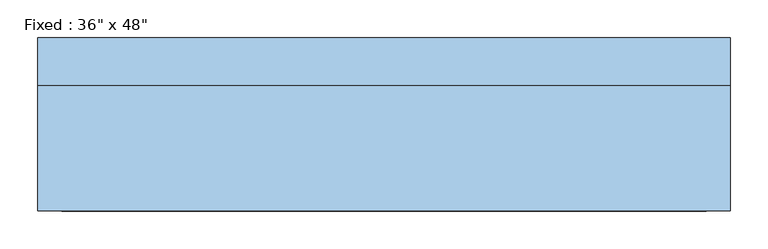
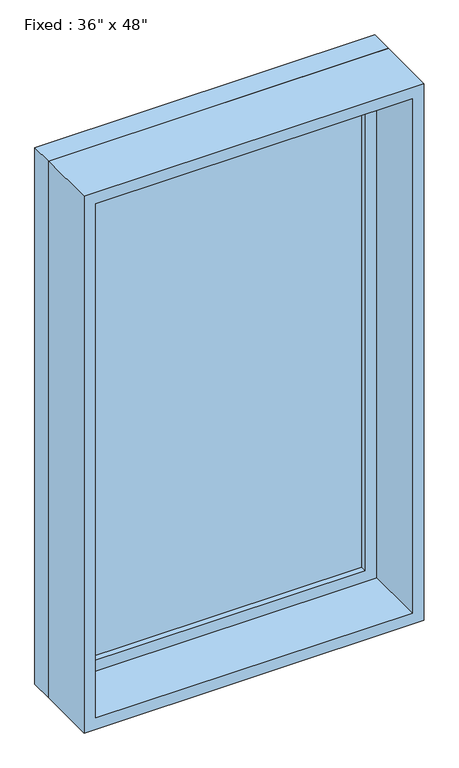
"""IFC4 building model written with IfcOpenShell, lengths in millimetres: window geometry."""

from ifc_helpers import new_model, si_unit, frame, origin, place, context, project, spatial, polyline, outline, extrude, source, transform, mapped, element, save


def window_cd393ee1(model_context):
    return source(origin(), model_context, "Body", "SweptSolid", [
        extrude(outline(polyline([(355.6, 66.675), (-431.8, 66.675), (-431.8, 79.375), (355.6, 79.375), (355.6, 66.675)])), frame((0.0, 0.0, 977.9), z_axis=(0.0, 0.0, 1.0), x_axis=(1.0, 0.0, 0.0)), (0.0, 0.0, 1.0), 1397.0),
        extrude(outline(polyline([(2419.35, -476.25), (933.45, -476.25), (933.45, 400.05), (2419.35, 400.05), (2419.35, -476.25)]), holes=[polyline([(2374.9, -431.8), (2374.9, 355.6), (977.9, 355.6), (977.9, -431.8), (2374.9, -431.8)])]), frame((0.0, 50.8, 0.0), z_axis=(0.0, 1.0, 0.0), x_axis=(0.0, 0.0, 1.0)), (0.0, 0.0, 1.0), 44.45),
        extrude(outline(polyline([(2438.4, -495.3), (914.4, -495.3), (914.4, 419.1), (2438.4, 419.1), (2438.4, -495.3)]), holes=[polyline([(2406.65, -463.55), (2406.65, 387.35), (946.15, 387.35), (946.15, -463.55), (2406.65, -463.55)])]), frame((0.0, -114.3, 0.0), z_axis=(0.0, 1.0, 0.0), x_axis=(0.0, 0.0, 1.0)), (0.0, 0.0, 1.0), 165.1),
        extrude(outline(polyline([(2438.4, 419.1), (2438.4, -495.3), (914.4, -495.3), (914.4, 419.1), (2438.4, 419.1)]), holes=[polyline([(2419.35, 400.05), (933.45, 400.05), (933.45, -476.25), (2419.35, -476.25), (2419.35, 400.05)])]), frame((0.0, 50.8, 0.0), z_axis=(0.0, 1.0, 0.0), x_axis=(0.0, 0.0, 1.0)), (0.0, 0.0, 1.0), 63.5),
    ])


if __name__ == "__main__":
    model = new_model("IFC4")
    model_context = context("Model", 3, world=origin())
    ifc_project = project(units=[si_unit("LENGTHUNIT", "METRE", prefix="MILLI")], contexts=[model_context])
    site = spatial("IfcSite", under=ifc_project)
    building = spatial("IfcBuilding", under=site)
    placement = place(None, origin())
    window_shape = window_cd393ee1(model_context)
    element("IfcWindow", 1, ObjectType="Fixed : 36\" x 48\"", at=placement, inside=building, context=model_context, shape_type="MappedRepresentation", body=[
        mapped(window_shape, transform((0.0, 0.0, 0.0), x_axis=(1.0, 0.0, 0.0), y_axis=(0.0, 1.0, 0.0), z_axis=(0.0, 0.0, 1.0))),
    ])
    save(model, "model.ifc")

# Revit data of these elements
# Type "Fixed : 36\" x 48\""
#   Type Mark = "1"
#   Construction Type Id = "GSP4R"
#   Assembly Code = "B2020100"
#   Analytic Construction = "1/8 in Pilkington single glazing"
#   Visual Light Transmittance = 0.9
#   Solar Heat Gain Coefficient = 0.78
#   Heat Transfer Coefficient (U) = 0.6496 BTU/(h·ft²·°F)
#   Height = 5' - 0"
#   Default Sill Height = 3' - 0"
#   Width = 3' - 0"
#   Window Inset = 0' - 0 3/4"
#   Define Thermal Properties by = 1
#   Define Thermal Properties by = 1
#   Glass Pane Material = Glass
#   Sash Material = Sash
#   Wall Closure = (empty or 0)
# Element 1 (IfcWindow, "Fixed : 36\" x 48\"")
#   Materials on its faces: "Sash", "Glass"
# Materials
#   "Glass": class "Glass", colour RGB 0 128 192, transparency 0.75, Description = "Soda Lime Glass", Cost = 0
#   "Sash": class "Wood", colour RGB 224 178 126, transparency 0, Cost = 0
